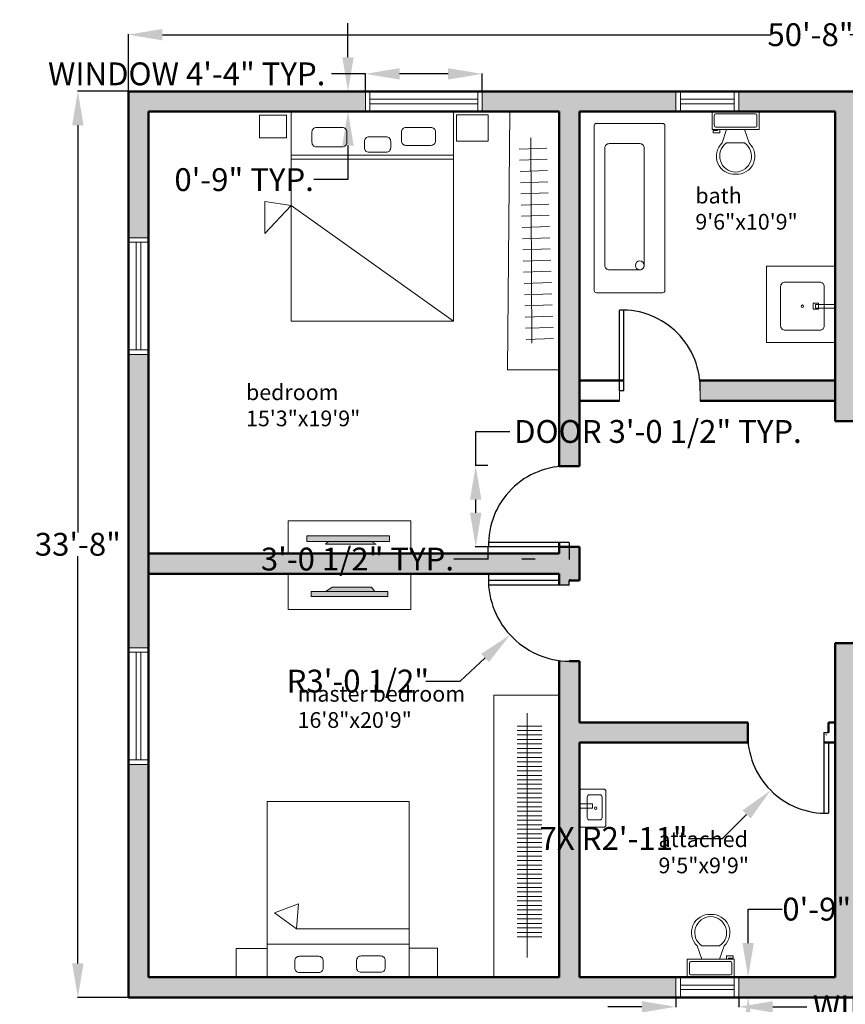
# Model space of a CAD drawing. Units: inches. Extents: x -2 to 7298, y -2 to 4583.
# Tile 4 of 6: x 6016 to 6384, y 4144 to 4583. Entities that reach past the tile are written whole.
import ezdxf

# ---------------------------------------------------------------- set-up
doc = ezdxf.new("R2010")
doc.units = ezdxf.units.IN
doc.header["$MEASUREMENT"] = 0
doc.linetypes.add('ACAD_ISO02W100', pattern=[15, 12, -3])
for name, color, linetype, lineweight in [('A-ANNO-DIMS', 2, 'Continuous', 18), ('A-AREA-IDEN', 7, 'Continuous', 18), ('A-DOOR', 4, 'Continuous', 25), ('A-FLOR-CASE', 30, 'Continuous', 18), ('A-FLOR-FIXT', 9, 'Continuous', 18), ('A-FURN', 8, 'Continuous', 18), ('A-FURN-PATT', 18, 'Continuous', 13), ('A-GLAZ', 4, 'Continuous', 18), ('A-WALL', 7, 'Continuous', 50), ('A-WALL-HIDN', 7, 'ACAD_ISO02W100', 18), ('A-WALL-PATT', 18, 'Continuous', 13)]:
    doc.layers.add(name, color=color, linetype=linetype, lineweight=lineweight)
doc.styles.get("Standard").update_dxf_attribs({"font": 'arial.ttf'})
doc.dimstyles.get("Standard").update_dxf_attribs({"dimtxt": 10.18, "dimasz": 15.18, "dimexe": 0.18, "dimexo": 0.0625, "dimgap": 0.09, "dimtad": 0, "dimtih": 1, "dimtoh": 1, "dimdec": 0, "dimzin": 0, "dimdsep": 46, "dimlunit": 3, "dimtxsty": 'Standard', "dimcen": 0.09, "dimadec": 0, "dimazin": 0, "dimtfac": 1, "dimtdec": 0, "dimtofl": 0, "dimtmove": 0, "dimatfit": 3, "dimfxl": 1, "dimtolj": 1, "dimtzin": 0, "dimarcsym": 0})

# ---------------------------------------------------------------- blocks, each defined once
blk = doc.blocks.new('*U4')
for p, q in [((9.5, -6), (9.5, -2)), ((-10, -8.5), (-8, -8.5)), ((-10, -9.5), (-10, -8.5)), ((-8, -8.5), (-8, -8)), ((-7, -8), (-7, -9.5)), ((-4, -8), (-6, -14)), ((4, -8), (6, -14)), ((-7, -9.5), (-10, -9.5)), ((4, -14), (-4, -14))]:
    blk.add_line(p, q)
blk.add_lwpolyline([(10.5, -8), (10.5, 0), (-10.5, 0), (-10.5, -8)], close=True)
for points in [[(-9.5, -2), (-9.5, -6)], [(8.5, -1), (-8.5, -1)], [(-8.5, -7), (8.5, -7)]]:
    blk.add_lwpolyline(points)
for centre, radius, start, end in [((-8.625, -1.875), 0.8839, 81.8699, 188.1301), ((8.625, -1.875), 0.8839, 351.8699, 98.1301), ((-8.625, -6.125), 0.8839, 171.869898, 278.1301), ((8.625, -6.125), 0.8839, 261.8699, 8.1301), ((-0.4772, -19.9188), 8.0953, 133.01722, 273.38), ((0.0374, -19.8731), 7.127, 124.50543, 269.7), ((-0.0373, -19.8731), 7.127, 270.3, 55.4946), ((0.4773, -19.9188), 8.0953, 266.62, 46.9828)]:
    blk.add_arc(centre, radius, start, end)
blk = doc.blocks.new('*D5')
at = {"layer": 'A-ANNO-DIMS', "color": 0, "lineweight": -2, "transparency": 16777216}
for p, q in [((6064.27, 4551.54), (6064.27, 4576.93)), ((6079.45, 4576.75), (6350.69, 4576.75)), ((6657.09, 4576.75), (6385.84, 4576.75)), ((6672.27, 4551.54), (6672.27, 4576.93))]:
    blk.add_line(p, q, dxfattribs=at)
at = {"layer": 'A-ANNO-DIMS', "color": 0, "transparency": 16777216}
for points in [[(6079.45, 4579.28), (6079.45, 4574.22), (6064.27, 4576.75)], [(6657.09, 4579.28), (6657.09, 4574.22), (6672.27, 4576.75)]]:
    blk.add_solid(points, dxfattribs=at)
at = {"layer": 'Defpoints', "color": 0, "transparency": 16777216}
for p in [(6672.27, 4576.75), (6064.27, 4551.48), (6672.27, 4551.48)]:
    blk.add_point(p, dxfattribs=at)
at = {"layer": 'A-ANNO-DIMS', "color": 0, "transparency": 16777216, "insert": (6368.27, 4576.75), "char_height": 10.18, "attachment_point": 5}
blk.add_mtext('\\A1;50\'-8"', dxfattribs=at)
blk = doc.blocks.new('*D6')
at = {"layer": 'A-ANNO-DIMS', "color": 0, "lineweight": -2, "transparency": 16777216}
for p, q in [((6064.2, 4551.54), (6041.55, 4551.54)), ((6041.73, 4536.36), (6041.73, 4354.8)), ((6041.73, 4162.66), (6041.73, 4344.22)), ((6064.2, 4147.48), (6041.55, 4147.48))]:
    blk.add_line(p, q, dxfattribs=at)
at = {"layer": 'A-ANNO-DIMS', "color": 0, "transparency": 16777216}
for points in [[(6039.2, 4536.36), (6044.26, 4536.36), (6041.73, 4551.54)], [(6039.2, 4162.66), (6044.26, 4162.66), (6041.73, 4147.48)]]:
    blk.add_solid(points, dxfattribs=at)
at = {"layer": 'Defpoints', "color": 0, "transparency": 16777216}
for p in [(6064.27, 4551.54), (6041.73, 4147.48), (6064.27, 4147.48)]:
    blk.add_point(p, dxfattribs=at)
at = {"layer": 'A-ANNO-DIMS', "color": 0, "transparency": 16777216, "insert": (6041.73, 4349.51), "char_height": 10.18, "attachment_point": 5}
blk.add_mtext('\\A1;33\'-8"', dxfattribs=at)
blk = doc.blocks.new('WINDOW-48IN')
for p, q in [((-2, 4.5), (-2, -4.5)), ((0, 4.5), (0, -4.5)), ((48, 4.5), (48, -4.5)), ((50, 4.5), (50, -4.5)), ((0, 1), (48, 1)), ((0, -1), (48, -1))]:
    blk.add_line(p, q)
blk = doc.blocks.new('WINDOW-24IN')
for p, q in [((-26, 4.5), (-26, -4.5)), ((-24, 4.5), (-24, -4.5)), ((0, 4.5), (0, -4.5)), ((2, 4.5), (2, -4.5)), ((-24, 1), (0, 1)), ((-24, -1), (0, -1))]:
    blk.add_line(p, q)
blk = doc.blocks.new('DOOR-SWING-36IN')
for p, q in [((0, 0), (0, 36)), ((2, 0), (2, 36)), ((2, 0), (0, 0))]:
    blk.add_line(p, q)
blk.add_arc((1, 1), 35.01, 358.3634, 91.6366)
blk = doc.blocks.new('*D35')
at = {"layer": 'A-ANNO-DIMS', "color": 0, "lineweight": -2, "transparency": 16777216}
for p, q in [((6169.92, 4559.28), (6154.74, 4559.28)), ((6169.92, 4551.54), (6169.92, 4559.46)), ((6206.74, 4559.28), (6185.1, 4559.28)), ((6221.92, 4551.54), (6221.92, 4559.46))]:
    blk.add_line(p, q, dxfattribs=at)
at = {"layer": 'A-ANNO-DIMS', "color": 0, "transparency": 16777216}
for points in [[(6185.1, 4561.81), (6185.1, 4556.75), (6169.92, 4559.28)], [(6206.74, 4561.81), (6206.74, 4556.75), (6221.92, 4559.28)]]:
    blk.add_solid(points, dxfattribs=at)
at = {"layer": 'Defpoints', "color": 0, "transparency": 16777216}
for p in [(6169.92, 4559.28), (6169.92, 4551.48), (6221.92, 4551.48)]:
    blk.add_point(p, dxfattribs=at)
at = {"layer": 'A-ANNO-DIMS', "color": 0, "transparency": 16777216, "insert": (6090.24, 4559.28), "char_height": 10.18, "attachment_point": 5}
blk.add_mtext('\\A1;WINDOW 4\'-4" TYP.', dxfattribs=at)
blk = doc.blocks.new('*D36')
at = {"layer": 'A-ANNO-DIMS', "color": 0, "lineweight": -2, "transparency": 16777216}
for p, q in [((6162.12, 4566.66), (6162.12, 4581.84)), ((6169.86, 4551.48), (6161.94, 4551.48)), ((6169.86, 4542.48), (6161.94, 4542.48)), ((6162.12, 4527.3), (6162.12, 4512.12)), ((6162.12, 4512.12), (6146.94, 4512.12))]:
    blk.add_line(p, q, dxfattribs=at)
at = {"layer": 'A-ANNO-DIMS', "color": 0, "transparency": 16777216}
for points in [[(6159.59, 4566.66), (6164.65, 4566.66), (6162.12, 4551.48)], [(6159.59, 4527.3), (6164.65, 4527.3), (6162.12, 4542.48)]]:
    blk.add_solid(points, dxfattribs=at)
at = {"layer": 'Defpoints', "color": 0, "transparency": 16777216}
for p in [(6169.92, 4551.48), (6162.12, 4542.48), (6169.92, 4542.48)]:
    blk.add_point(p, dxfattribs=at)
at = {"layer": 'A-ANNO-DIMS', "color": 0, "transparency": 16777216, "insert": (6115.83, 4512.12), "char_height": 10.18, "attachment_point": 5}
blk.add_mtext('\\A1;0\'-9" TYP.', dxfattribs=at)
blk = doc.blocks.new('*D39')
at = {"layer": 'A-ANNO-DIMS', "color": 0, "lineweight": -2, "transparency": 16777216}
for p, q in [((6308.27, 4147.41), (6308.27, 4143.1)), ((6336.27, 4147.41), (6336.27, 4143.1)), ((6293.09, 4143.28), (6277.91, 4143.28)), ((6351.45, 4143.28), (6366.63, 4143.28))]:
    blk.add_line(p, q, dxfattribs=at)
at = {"layer": 'A-ANNO-DIMS', "color": 0, "transparency": 16777216}
for points in [[(6293.09, 4145.81), (6293.09, 4140.75), (6308.27, 4143.28)], [(6351.45, 4145.81), (6351.45, 4140.75), (6336.27, 4143.28)]]:
    blk.add_solid(points, dxfattribs=at)
at = {"layer": 'Defpoints', "color": 0, "transparency": 16777216}
for p in [(6308.27, 4147.48), (6336.27, 4147.48), (6336.27, 4143.28)]:
    blk.add_point(p, dxfattribs=at)
at = {"layer": 'A-ANNO-DIMS', "color": 0, "transparency": 16777216, "insert": (6431.13, 4143.28), "char_height": 10.18, "attachment_point": 5}
blk.add_mtext('\\A1;WINDOW 2\'-4" TYP.', dxfattribs=at)
blk = doc.blocks.new('*D40')
at = {"layer": 'A-ANNO-DIMS', "color": 0, "lineweight": -2, "transparency": 16777216}
for p, q in [((6340.47, 4171.66), (6340.47, 4186.84)), ((6340.47, 4186.84), (6355.65, 4186.84)), ((6336.33, 4156.48), (6340.65, 4156.48)), ((6336.33, 4147.48), (6340.65, 4147.48)), ((6340.47, 4132.3), (6340.47, 4117.12))]:
    blk.add_line(p, q, dxfattribs=at)
at = {"layer": 'A-ANNO-DIMS', "color": 0, "transparency": 16777216}
for points in [[(6337.94, 4171.66), (6343, 4171.66), (6340.47, 4156.48)], [(6337.94, 4132.3), (6343, 4132.3), (6340.47, 4147.48)]]:
    blk.add_solid(points, dxfattribs=at)
at = {"layer": 'Defpoints', "color": 0, "transparency": 16777216}
for p in [(6336.27, 4156.48), (6340.47, 4156.48), (6336.27, 4147.48)]:
    blk.add_point(p, dxfattribs=at)
at = {"layer": 'A-ANNO-DIMS', "color": 0, "transparency": 16777216, "insert": (6386.76, 4186.84), "char_height": 10.18, "attachment_point": 5}
blk.add_mtext('\\A1;0\'-9" TYP.', dxfattribs=at)
blk = doc.blocks.new('*D41')
at = {"layer": 'A-ANNO-DIMS', "color": 0, "lineweight": -2, "transparency": 16777216}
for p, q in [((6219.05, 4384.64), (6219.05, 4399.82)), ((6219.05, 4399.82), (6234.23, 4399.82)), ((6224.43, 4384.64), (6218.87, 4384.64)), ((6219.05, 4363.54), (6219.05, 4369.46)), ((6224.43, 4348.36), (6218.87, 4348.36))]:
    blk.add_line(p, q, dxfattribs=at)
at = {"layer": 'A-ANNO-DIMS', "color": 0, "transparency": 16777216}
for points in [[(6216.52, 4369.46), (6221.58, 4369.46), (6219.05, 4384.64)], [(6216.52, 4363.54), (6221.58, 4363.54), (6219.05, 4348.36)]]:
    blk.add_solid(points, dxfattribs=at)
at = {"layer": 'Defpoints', "color": 0, "transparency": 16777216}
for p in [(6219.05, 4384.64), (6224.49, 4384.64), (6224.49, 4348.36)]:
    blk.add_point(p, dxfattribs=at)
at = {"layer": 'A-ANNO-DIMS', "color": 0, "transparency": 16777216, "insert": (6300.26, 4399.82), "char_height": 10.18, "attachment_point": 5}
blk.add_mtext('\\A1;DOOR 3\'-0 1/2" TYP.', dxfattribs=at)
blk = doc.blocks.new('*D42')
at = {"layer": 'A-ANNO-DIMS', "color": 0, "lineweight": -2, "transparency": 16777216}
for p, q in [((6224.49, 4348.3), (6224.49, 4342.74)), ((6260.77, 4348.3), (6260.77, 4342.74)), ((6224.49, 4342.92), (6209.31, 4342.92)), ((6245.59, 4342.92), (6239.67, 4342.92))]:
    blk.add_line(p, q, dxfattribs=at)
at = {"layer": 'A-ANNO-DIMS', "color": 0, "transparency": 16777216}
for points in [[(6239.67, 4345.45), (6239.67, 4340.39), (6224.49, 4342.92)], [(6245.59, 4345.45), (6245.59, 4340.39), (6260.77, 4342.92)]]:
    blk.add_solid(points, dxfattribs=at)
at = {"layer": 'Defpoints', "color": 0, "transparency": 16777216}
for p in [(6224.49, 4348.36), (6260.77, 4348.36), (6224.49, 4342.92)]:
    blk.add_point(p, dxfattribs=at)
at = {"layer": 'A-ANNO-DIMS', "color": 0, "transparency": 16777216, "insert": (6166.34, 4342.92), "char_height": 10.18, "attachment_point": 5}
blk.add_mtext('\\A1;3\'-0 1/2" TYP.', dxfattribs=at)
blk = doc.blocks.new('*D66')
at = {"layer": 'A-ANNO-DIMS', "color": 0, "lineweight": -2, "transparency": 16777216}
for p, q in [((6030.986562, 4134.626544), (6015.806562, 4134.626544)), ((6046.166562, 4097.966533), (6046.166562, 4134.806544)), ((6112.578072, 4097.966533), (6112.578072, 4134.806544)), ((6127.758072, 4134.626544), (6142.938072, 4134.626544))]:
    blk.add_line(p, q, dxfattribs=at)
at = {"layer": 'A-ANNO-DIMS', "color": 0, "transparency": 16777216}
for points in [[(6030.986562, 4137.156544), (6030.986562, 4132.096544), (6046.166562, 4134.626544)], [(6127.758072, 4137.156544), (6127.758072, 4132.096544), (6112.578072, 4134.626544)]]:
    blk.add_solid(points, dxfattribs=at)
at = {"layer": 'Defpoints', "color": 0, "transparency": 16777216}
for p in [(6112.578072, 4134.626544), (6046.166562, 4097.904033), (6112.578072, 4097.904033)]:
    blk.add_point(p, dxfattribs=at)
at = {"layer": 'A-ANNO-DIMS', "color": 0, "transparency": 16777216, "insert": (6079.372317, 4134.626544), "char_height": 10.18, "attachment_point": 5}
blk.add_mtext('\\A1;5\'-6 1/2"', dxfattribs=at)
blk = doc.blocks.new('*D92')
at = {"layer": 'A-ANNO-DIMS', "color": 0, "lineweight": -2, "transparency": 16777216}
for p, q in [((6261.09, 4333.86), (6261.27, 4333.86)), ((6261.18, 4333.77), (6261.18, 4333.95)), ((6212.05, 4288.51), (6223.21, 4298.81)), ((6196.87, 4288.51), (6212.05, 4288.51))]:
    blk.add_line(p, q, dxfattribs=at)
at = {"layer": 'A-ANNO-DIMS', "color": 0, "transparency": 16777216}
blk.add_solid([(6221.49, 4300.67), (6224.92, 4296.95), (6234.36, 4309.1)], dxfattribs=at)
at = {"layer": 'Defpoints', "color": 0, "transparency": 16777216}
for p in [(6261.18, 4333.86), (6234.36, 4309.1)]:
    blk.add_point(p, dxfattribs=at)
at = {"layer": 'A-ANNO-DIMS', "color": 0, "transparency": 16777216, "insert": (6166.52, 4288.51), "char_height": 10.18, "attachment_point": 5}
blk.add_mtext('\\A1;R3\'-0 1/2"', dxfattribs=at)
blk = doc.blocks.new('*D93')
at = {"layer": 'A-ANNO-DIMS', "color": 0, "lineweight": -2, "transparency": 16777216}
for p, q in [((6375.18, 4264.57), (6375.36, 4264.57)), ((6375.27, 4264.48), (6375.27, 4264.66)), ((6329.04, 4218.34), (6339.77, 4229.08)), ((6313.86, 4218.34), (6329.04, 4218.34))]:
    blk.add_line(p, q, dxfattribs=at)
at = {"layer": 'A-ANNO-DIMS', "color": 0, "transparency": 16777216}
blk.add_solid([(6337.99, 4230.87), (6341.56, 4227.29), (6350.51, 4239.81)], dxfattribs=at)
at = {"layer": 'Defpoints', "color": 0, "transparency": 16777216}
for p in [(6375.27, 4264.57), (6350.51, 4239.81)]:
    blk.add_point(p, dxfattribs=at)
at = {"layer": 'A-ANNO-DIMS', "color": 0, "transparency": 16777216, "insert": (6280.52, 4218.34), "char_height": 10.18, "attachment_point": 5}
blk.add_mtext('\\A1;7X R2\'-11"', dxfattribs=at)

msp = doc.modelspace()

# ---------------------------------------------------------------- hatches: boundary and pattern name
at = {"layer": 'A-FURN-PATT'}
h = msp.add_hatch(color=256, dxfattribs=at)
h.dxf.hatch_style = 1
h.paths.add_polyline_path([(6180.61, 4353.29), (6143.73, 4353.29), (6143.73, 4350.76), (6180.61, 4350.76)])
h.paths.add_polyline_path([(6172.61, 4350.76), (6153.4, 4350.76), (6152.16, 4349.62), (6174.65, 4349.62)])
h = msp.add_hatch(color=256, dxfattribs=at)
h.dxf.hatch_style = 1
h.paths.add_polyline_path([(6179.95, 4328.53), (6145.73, 4328.53), (6145.73, 4326.18), (6179.95, 4326.18)])
h.paths.add_polyline_path([(6172.57, 4330.32), (6155.12, 4330.32), (6152.28, 4328.53), (6174.06, 4328.53)])
at = {"layer": 'A-WALL-PATT'}
h = msp.add_hatch(color=256, dxfattribs=at)
h.dxf.hatch_style = 1
h.paths.add_polyline_path([(6073.27, 4434.19), (6064.27, 4434.19), (6064.27, 4303.39), (6073.27, 4303.39), (6073.27, 4305.48)])
h.paths.add_polyline_path([(6265.27, 4348.36), (6256.27, 4348.36), (6256.27, 4345.36), (6073.27, 4345.36), (6073.27, 4336.36), (6256.27, 4336.36), (6256.27, 4331.36), (6260.77, 4331.36), (6260.77, 4333.36), (6265.27, 4333.36)])
h.paths.add_polyline_path([(6073.27, 4251.39), (6064.27, 4251.39), (6064.27, 4147.48), (6308.27, 4147.48), (6308.27, 4156.48), (6265.27, 4156.48), (6265.27, 4256.48), (6265.27, 4261.07), (6340.27, 4261.07), (6340.27, 4263.57, -0.014283), (6340.27, 4265.57), (6340.27, 4270.07), (6265.27, 4270.07), (6265.27, 4297.36), (6261.6, 4297.36, -0.036646), (6256.27, 4297.69), (6256.27, 4156.48), (6073.27, 4156.48)])
h.paths.add_polyline_path([(6422.77, 4156.48), (6388.27, 4156.48), (6388.27, 4305.48), (6379.27, 4305.48), (6379.27, 4270.07), (6379.27, 4261.07), (6379.27, 4156.48), (6336.27, 4156.48), (6336.27, 4147.48), (6422.77, 4147.48)])
h.paths.add_polyline_path([(6552.77, 4156.48), (6518.27, 4156.48), (6518.27, 4261.05), (6509.27, 4261.05), (6509.27, 4156.48), (6474.77, 4156.48), (6474.77, 4147.48), (6552.77, 4147.48)])
h.paths.add_polyline_path([(6672.27, 4252.66), (6663.27, 4252.66), (6663.27, 4156.48), (6628.77, 4156.48), (6628.77, 4147.48), (6672.27, 4147.48)])
h.paths.add_polyline_path([(6672.27, 4385.98), (6663.27, 4385.98), (6663.27, 4305.48), (6561.68, 4305.48, -0.01877), (6561.79, 4302.48), (6561.79, 4296.48), (6663.27, 4296.48), (6663.27, 4287.22), (6672.27, 4287.22)])
h.paths.add_polyline_path([(6518.27, 4542.48), (6663.27, 4542.48), (6663.27, 4461.98), (6672.27, 4461.98), (6672.27, 4551.48), (6336.27, 4551.48), (6336.27, 4542.48), (6379.27, 4542.48), (6379.27, 4404.48), (6388.27, 4404.48), (6388.27, 4506.48), (6388.27, 4542.48), (6509.27, 4542.48), (6509.27, 4413.48), (6509.27, 4404.48), (6509.27, 4305.48), (6518.27, 4305.48)])
h.paths.add_polyline_path([(6379.27, 4422.48), (6319.12, 4422.48), (6319.12, 4419.98, -0.014283), (6319.12, 4417.98), (6319.12, 4413.48), (6379.27, 4413.48)])
h.paths.add_polyline_path([(6265.27, 4542.48), (6308.27, 4542.48), (6308.27, 4551.48), (6221.92, 4551.48), (6221.92, 4542.48), (6256.27, 4542.48), (6256.27, 4384.36), (6258.77, 4384.36, -0.014283), (6260.77, 4384.36), (6265.27, 4384.36)])
h.paths.add_polyline_path([(6169.92, 4551.48), (6064.27, 4551.48), (6064.27, 4486.19), (6073.27, 4486.19), (6073.27, 4542.48), (6169.92, 4542.48)])

# ---------------------------------------------------------------- linework, layer by layer
at = {"layer": 'A-DOOR'}
for p, q in [((6256.27, 4333.36), (6224.77, 4333.36)), ((6260.77, 4331.36), (6260.77, 4333.36)), ((6260.77, 4331.36), (6224.77, 4331.36)), ((6374.27, 4265.57), (6374.27, 4229.57)), ((6374.27, 4265.57), (6376.27, 4265.57)), ((6376.27, 4261.07), (6376.27, 4229.57))]:
    msp.add_line(p, q, dxfattribs=at)
for centre, radius, start, end in [((6261.18, 4333.86), 36.5, 176.0728, 269.346), ((6375.27, 4264.57), 35.01, 178.3634, 271.6366)]:
    msp.add_arc(centre, radius, start, end, dxfattribs=at)
at = {"layer": 'A-FLOR-CASE'}
for p, q in [((6234.29, 4542.48), (6233.25, 4427.35)), ((6243.67, 4530.72), (6244.02, 4439.15)), ((6238.44, 4525.75), (6250.68, 4526.19)), ((6238.62, 4520.76), (6250.85, 4521.19)), ((6238.8, 4515.76), (6251.03, 4516.2)), ((6238.98, 4510.76), (6251.21, 4511.2)), ((6239.16, 4505.77), (6251.39, 4506.2)), ((6239.34, 4500.77), (6251.57, 4501.21)), ((6239.51, 4495.77), (6251.75, 4496.21)), ((6239.69, 4490.78), (6251.92, 4491.21)), ((6239.87, 4485.78), (6252.1, 4486.22)), ((6240.05, 4480.78), (6252.28, 4481.22)), ((6240.23, 4475.79), (6252.46, 4476.22)), ((6240.41, 4470.79), (6252.64, 4471.23)), ((6240.58, 4465.79), (6252.81, 4466.23)), ((6240.76, 4460.8), (6252.99, 4461.23)), ((6240.94, 4455.8), (6253.17, 4456.24)), ((6241.12, 4450.8), (6253.35, 4451.24)), ((6241.3, 4445.81), (6253.53, 4446.24)), ((6241.47, 4440.81), (6253.71, 4441.25)), ((6233.25, 4427.35), (6256.27, 4427.35)), ((6256.27, 4282.25), (6227.05, 4282.25)), ((6227.05, 4282.25), (6227.05, 4156.48)), ((6241.97, 4274.22), (6241.97, 4165.31)), ((6237.54, 4268.48), (6248.51, 4268.48)), ((6237.54, 4266.48), (6248.51, 4266.48)), ((6237.54, 4264.48), (6248.51, 4264.48)), ((6237.54, 4262.48), (6248.51, 4262.48)), ((6237.54, 4260.48), (6248.51, 4260.48)), ((6237.54, 4258.48), (6248.51, 4258.48)), ((6237.54, 4256.48), (6248.51, 4256.48)), ((6237.54, 4254.48), (6248.51, 4254.48)), ((6237.54, 4252.48), (6248.51, 4252.48)), ((6237.54, 4250.48), (6248.51, 4250.48)), ((6237.54, 4248.48), (6248.51, 4248.48)), ((6237.54, 4246.48), (6248.51, 4246.48)), ((6237.54, 4244.48), (6248.51, 4244.48)), ((6237.54, 4242.48), (6248.51, 4242.48)), ((6237.54, 4240.48), (6248.51, 4240.48)), ((6237.54, 4238.48), (6248.51, 4238.48)), ((6237.54, 4236.48), (6248.51, 4236.48)), ((6237.54, 4234.48), (6248.51, 4234.48)), ((6237.54, 4232.48), (6248.51, 4232.48)), ((6237.54, 4230.48), (6248.51, 4230.48)), ((6237.54, 4228.48), (6248.51, 4228.48)), ((6237.54, 4226.48), (6248.51, 4226.48)), ((6237.54, 4224.48), (6248.51, 4224.48)), ((6237.54, 4222.48), (6248.51, 4222.48)), ((6237.54, 4220.48), (6248.51, 4220.48)), ((6237.54, 4218.48), (6248.51, 4218.48)), ((6237.54, 4216.48), (6248.51, 4216.48)), ((6237.54, 4214.48), (6248.51, 4214.48)), ((6237.54, 4212.48), (6248.51, 4212.48)), ((6237.54, 4210.48), (6248.51, 4210.48)), ((6237.54, 4208.48), (6248.51, 4208.48)), ((6237.54, 4206.48), (6248.51, 4206.48)), ((6237.54, 4204.48), (6248.51, 4204.48)), ((6237.54, 4202.48), (6248.51, 4202.48)), ((6237.54, 4200.48), (6248.51, 4200.48)), ((6237.54, 4198.48), (6248.51, 4198.48)), ((6237.54, 4196.48), (6248.51, 4196.48)), ((6237.54, 4194.48), (6248.51, 4194.48)), ((6237.54, 4192.48), (6248.51, 4192.48)), ((6237.54, 4190.48), (6248.51, 4190.48)), ((6237.54, 4188.48), (6248.51, 4188.48)), ((6237.54, 4186.48), (6248.51, 4186.48)), ((6237.54, 4184.48), (6248.51, 4184.48)), ((6237.54, 4182.48), (6248.51, 4182.48)), ((6237.54, 4180.48), (6248.51, 4180.48)), ((6237.54, 4178.48), (6248.51, 4178.48)), ((6237.54, 4176.48), (6248.51, 4176.48)), ((6237.54, 4174.48), (6248.51, 4174.48))]:
    msp.add_line(p, q, dxfattribs=at)
at = {"layer": 'A-FLOR-FIXT'}
for p, q in [((6379.27, 4456.45), (6370.45, 4456.45)), ((6370.45, 4456.45), (6370.45, 4454.87)), ((6370.45, 4454.87), (6379.27, 4454.87)), ((6265.27, 4233.71), (6265.27, 4233.71))]:
    msp.add_line(p, q, dxfattribs=at)
for points in [[(6271.87, 4536.16, -0.414214), (6272.87, 4537.16), (6302.4, 4537.16, -0.414214), (6303.4, 4536.16), (6303.4, 4462.68, -0.414214), (6302.4, 4461.68), (6272.87, 4461.68, -0.414214), (6271.87, 4462.68)], [(6276.57, 4526.16, -0.414214), (6278.57, 4528.16), (6292.19, 4528.16, -0.414214), (6294.19, 4526.16), (6294.19, 4473.84, -0.414214), (6292.19, 4471.84), (6278.57, 4471.84, -0.414214), (6276.57, 4473.84)], [(6354.95, 4464.41, -0.414214), (6356.95, 4466.41), (6372.42, 4466.41, -0.414214), (6374.42, 4464.41), (6374.42, 4446.98, -0.414214), (6372.42, 4444.98), (6356.95, 4444.98, -0.414214), (6354.95, 4446.98)], [(6265.27, 4239.35, -0.414214), (6266.27, 4240.35), (6276.07, 4240.35, -0.414214), (6277.07, 4239.35), (6277.07, 4224.37, -0.414214), (6276.07, 4223.37), (6266.27, 4223.37, -0.414214), (6265.27, 4224.37)], [(6268.72, 4236.81, -0.414214), (6269.72, 4237.81), (6274.37, 4237.81, -0.414214), (6275.37, 4236.81), (6275.37, 4227.61, -0.414214), (6274.37, 4226.61), (6269.72, 4226.61, -0.414214), (6268.72, 4227.61)]]:
    msp.add_lwpolyline(points, format="xyb", close=True, dxfattribs=at)
for points in [[(6379.27, 4473.48), (6379.27, 4473.48), (6348.59, 4473.48), (6348.59, 4473.48), (6348.59, 4439.42), (6348.59, 4439.42), (6379.27, 4439.42), (6379.27, 4439.42)], [(6369.44, 4456.99), (6369.44, 4456.99), (6371.82, 4456.99), (6371.82, 4456.99), (6371.82, 4454.31), (6371.82, 4454.31), (6369.44, 4454.31), (6369.44, 4454.31)], [(6265.27, 4233.71), (6265.27, 4233.71), (6271.17, 4233.71), (6271.17, 4233.71), (6271.17, 4231.86), (6271.17, 4231.86), (6265.27, 4231.86), (6265.27, 4231.86)]]:
    msp.add_lwpolyline(points, close=True, dxfattribs=at)
for centre, radius in [((6292.19, 4473.84), 2), ((6364.68, 4455.69), 0.525), ((6272.48, 4231.86), 0.544)]:
    msp.add_circle(centre, radius, dxfattribs=at)
at = {"layer": 'A-FURN'}
for p, q in [((6136.73, 4522.96), (6209.1, 4522.96)), ((6136.73, 4521.27), (6209.1, 4521.27)), ((6136.73, 4500.65), (6125.01, 4502.35)), ((6125.01, 4502.35), (6125.01, 4488.07)), ((6125.01, 4488.07), (6136.73, 4500.65)), ((6209.1, 4449), (6136.73, 4500.65)), ((6153.4, 4350.76), (6152.16, 4349.62)), ((6152.16, 4349.62), (6174.65, 4349.62)), ((6174.65, 4349.62), (6172.61, 4350.76)), ((6152.28, 4328.53), (6155.12, 4330.32)), ((6155.12, 4330.32), (6172.57, 4330.32)), ((6172.57, 4330.32), (6174.06, 4328.53)), ((6129.4, 4185.18), (6140.08, 4189.15)), ((6140.08, 4189.15), (6139.19, 4177.99)), ((6139.19, 4177.99), (6129.4, 4185.18)), ((6189.34, 4177.99), (6139.19, 4177.99)), ((6189.34, 4171.17), (6126.16, 4171.17))]:
    msp.add_line(p, q, dxfattribs=at)
for points in [[(6134.69, 4540.91), (6134.69, 4540.91), (6122.69, 4540.91), (6122.69, 4540.91), (6122.69, 4530.72), (6122.69, 4530.72), (6134.69, 4530.72), (6134.69, 4530.72)], [(6136.73, 4542.48), (6136.73, 4542.48), (6209.1, 4542.48), (6209.1, 4542.48), (6209.1, 4449), (6209.1, 4449), (6136.73, 4449), (6136.73, 4449)], [(6210.54, 4541.05), (6210.54, 4541.05), (6224.56, 4541.05), (6224.56, 4541.05), (6224.56, 4529.31), (6224.56, 4529.31), (6210.54, 4529.31), (6210.54, 4529.31)], [(6135.43, 4345.36), (6135.43, 4345.36), (6190.17, 4345.36), (6190.17, 4345.36), (6190.17, 4359.97), (6190.17, 4359.97), (6135.43, 4359.97), (6135.43, 4359.97)], [(6143.73, 4350.76), (6143.73, 4350.76), (6180.61, 4350.76), (6180.61, 4350.76), (6180.61, 4353.29), (6180.61, 4353.29), (6143.73, 4353.29), (6143.73, 4353.29)], [(6135.42, 4336.36), (6135.42, 4336.36), (6190.17, 4336.36), (6190.17, 4336.36), (6190.17, 4320.4), (6190.17, 4320.4), (6135.42, 4320.4), (6135.42, 4320.4)], [(6145.73, 4328.53), (6145.73, 4328.53), (6179.95, 4328.53), (6179.95, 4328.53), (6179.95, 4326.18), (6179.95, 4326.18), (6145.73, 4326.18), (6145.73, 4326.18)], [(6126.16, 4234.84), (6126.16, 4234.84), (6189.34, 4234.84), (6189.34, 4234.84), (6189.34, 4156.48), (6189.34, 4156.48), (6126.16, 4156.48), (6126.16, 4156.48)], [(6126.16, 4169.34), (6126.16, 4169.34), (6112.21, 4169.34), (6112.21, 4169.34), (6112.21, 4156.48), (6112.21, 4156.48), (6126.16, 4156.48), (6126.16, 4156.48)], [(6189.34, 4169.44), (6189.34, 4169.44), (6202.03, 4169.44), (6202.03, 4169.44), (6202.03, 4156.48), (6202.03, 4156.48), (6189.34, 4156.48), (6189.34, 4156.48)]]:
    msp.add_lwpolyline(points, close=True, dxfattribs=at)
for points in [[(6161.58, 4533.36, 0.414214), (6159.58, 4535.36), (6148.07, 4535.36, 0.414214), (6146.07, 4533.36), (6146.07, 4528.75, 0.414214), (6148.07, 4526.75), (6159.58, 4526.75, 0.414214), (6161.58, 4528.75)], [(6185.95, 4533.36, -0.414214), (6187.95, 4535.36), (6199.09, 4535.36, -0.414214), (6201.09, 4533.36), (6201.09, 4529.37, -0.414214), (6199.09, 4527.37), (6187.95, 4527.37, -0.414214), (6185.95, 4529.37)], [(6169.46, 4529.18, -0.414214), (6171.46, 4531.18), (6179.15, 4531.18, -0.414214), (6181.15, 4529.18), (6181.15, 4526.29, -0.414214), (6179.15, 4524.29), (6171.46, 4524.29, -0.414214), (6169.46, 4526.29)], [(6138.41, 4163.82, -0.414214), (6140.41, 4165.82), (6149.12, 4165.82, -0.414214), (6151.12, 4163.82), (6151.12, 4160.52, -0.414214), (6149.12, 4158.52), (6140.41, 4158.52, -0.414214), (6138.41, 4160.52)], [(6165.96, 4163.96, -0.414214), (6167.96, 4165.96), (6176.67, 4165.96, -0.414214), (6178.67, 4163.96), (6178.67, 4160.65, -0.414214), (6176.67, 4158.65), (6167.96, 4158.65, -0.414214), (6165.96, 4160.65)]]:
    msp.add_lwpolyline(points, format="xyb", close=True, dxfattribs=at)
at = {"layer": 'A-WALL'}
for p, q in [((6672.27, 4551.48), (6064.27, 4551.48)), ((6064.27, 4147.48), (6064.27, 4551.48)), ((6256.27, 4542.48), (6073.27, 4542.48)), ((6073.27, 4305.48), (6073.27, 4542.48)), ((6256.27, 4384.2), (6256.27, 4542.48)), ((6379.27, 4542.48), (6265.27, 4542.48)), ((6265.27, 4384.36), (6265.27, 4542.48)), ((6379.27, 4404.48), (6379.27, 4542.48)), ((6285.12, 4422.48), (6265.27, 4422.48)), ((6379.27, 4422.48), (6318.95, 4422.48)), ((6283.12, 4413.48), (6265.27, 4413.48)), ((6379.27, 4413.48), (6319.12, 4413.48)), ((6379.27, 4404.48), (6388.27, 4404.48)), ((6256.27, 4384.36), (6265.27, 4384.36)), ((6256.27, 4345.36), (6256.27, 4350.36)), ((6256.27, 4348.36), (6265.27, 4348.36)), ((6265.27, 4333.36), (6265.27, 4348.36)), ((6256.27, 4345.36), (6073.27, 4345.36)), ((6256.27, 4336.36), (6073.27, 4336.36)), ((6256.27, 4331.36), (6256.27, 4336.36)), ((6260.77, 4333.36), (6265.27, 4333.36)), ((6073.27, 4305.48), (6073.27, 4296.48)), ((6388.27, 4305.48), (6379.27, 4305.48)), ((6379.27, 4270.07), (6379.27, 4305.48)), ((6073.27, 4156.48), (6073.27, 4296.48)), ((6256.27, 4156.48), (6256.27, 4297.69)), ((6260.77, 4297.36), (6265.27, 4297.36)), ((6265.27, 4270.07), (6265.27, 4297.36)), ((6340.27, 4270.07), (6265.27, 4270.07)), ((6340.27, 4270.07), (6340.27, 4261.07)), ((6379.27, 4270.07), (6376.27, 4270.07)), ((6376.27, 4270.07), (6376.27, 4265.57)), ((6379.27, 4270.07), (6379.27, 4261.07)), ((6265.27, 4256.43), (6265.27, 4261.07)), ((6340.43, 4261.07), (6265.27, 4261.07)), ((6379.27, 4261.07), (6374.27, 4261.07)), ((6379.27, 4156.48), (6379.27, 4261.07)), ((6265.27, 4156.48), (6265.27, 4256.48)), ((6073.27, 4156.48), (6256.27, 4156.48)), ((6265.27, 4156.48), (6379.27, 4156.48)), ((6064.27, 4147.48), (6672.27, 4147.48))]:
    msp.add_line(p, q, dxfattribs=at)
at = {"layer": 'A-WALL-HIDN'}
for p, q in [((6283.12, 4422.48), (6283.12, 4413.48)), ((6319.12, 4422.48), (6319.12, 4413.48))]:
    msp.add_line(p, q, dxfattribs=at)

# ---------------------------------------------------------------- block references
at = {"layer": 'A-DOOR'}
msp.add_blockref('DOOR-SWING-36IN', (6283.12, 4417.98), dxfattribs=at)
at = {"layer": 'A-DOOR', "rotation": 90.00000000000146}
msp.add_blockref('DOOR-SWING-36IN', (6260.77, 4348.36), dxfattribs=at)
at = {"layer": 'A-FLOR-FIXT'}
msp.add_blockref('*U4', (6334.87, 4542.48), dxfattribs=at)
at = {"layer": 'A-FLOR-FIXT', "rotation": 180}
msp.add_blockref('*U4', (6323.77, 4156.48), dxfattribs=at)
at = {"layer": 'A-GLAZ'}
for p, rotation in [((6219.92, 4546.98), 180), ((6068.77, 4436.19), 90.0000000000016), ((6068.77, 4301.39), 270.0000000000055)]:
    msp.add_blockref('WINDOW-48IN', p, dxfattribs=dict(at, rotation=rotation))
for p in [(6334.27, 4546.98), (6334.27, 4151.98)]:
    msp.add_blockref('WINDOW-24IN', p, dxfattribs=at)

# ---------------------------------------------------------------- texts
at = {"layer": 'A-AREA-IDEN', "char_height": 7, "attachment_point": 1}
for s, insert in [('bath\\P9\'6"x10\'9"', (6316.93, 4508.49)), ('bedroom\\P15\'3"x19\'9"', (6116.68, 4420.81)), ('master bedroom\\P16\'8"x20\'9"', (6139.65, 4286.34)), ('attached\\P9\'5"x9\'9"', (6300.51, 4221.49))]:
    msp.add_mtext_dynamic_manual_height_columns(s, width=119.0967, gutter_width=1, heights=[0], dxfattribs=dict(at, insert=insert))

# ---------------------------------------------------------------- dimensions: what is measured, and where the dimension line sits
at = {"layer": 'A-ANNO-DIMS'}
for base, p1, p2, angle, text, picture, middle in [((6169.92, 4559.28), (6221.92, 4551.48), (6169.92, 4551.48), 180, 'WINDOW <> TYP.', '*D35', (6090.24, 4559.28)), ((6162.12, 4542.48), (6169.92, 4551.48), (6169.92, 4542.48), 270, '<> TYP.', '*D36', (6115.83, 4512.12)), ((6219.05, 4384.64), (6224.49, 4348.36), (6224.49, 4384.64), 90, 'DOOR <> TYP.', '*D41', (6300.26, 4399.82)), ((6224.49, 4342.92), (6260.77, 4348.36), (6224.49, 4348.36), 180, '<> TYP.', '*D42', (6166.34, 4342.92)), ((6340.47, 4156.48), (6336.27, 4147.48), (6336.27, 4156.48), 90, '<> TYP.', '*D40', (6386.76, 4186.84))]:
    dim = msp.add_linear_dim(base=base, p1=p1, p2=p2, angle=angle, text=text, dimstyle='Standard', override={"dimdec": 1, "dimlfac": 1, "dimrnd": 0, "dimzin": 1, "dimdsep": 46, "dimlunit": 4, "dimfrac": 2}, dxfattribs=at)
    dim.commit()
    dim.dimension.update_dxf_attribs({"geometry": picture, "text_midpoint": middle})
for base, p1, p2, override, picture, middle in [((6672.27, 4576.75), (6064.27, 4551.48), (6672.27, 4551.48), {"dimclrd": 0, "dimclre": 0, "dimclrt": 0}, '*D5', (6368.27, 4576.75)), ((6112.58, 4134.63), (6046.17, 4097.9), (6112.58, 4097.9), {"dimdec": 1, "dimlfac": 1, "dimrnd": 0, "dimzin": 1, "dimdsep": 46, "dimlunit": 4, "dimfrac": 2}, '*D66', (6079.37, 4134.63))]:
    dim = msp.add_linear_dim(base=base, p1=p1, p2=p2, dimstyle='Standard', override=override, dxfattribs=at)
    dim.commit()
    dim.dimension.update_dxf_attribs({"geometry": picture, "text_midpoint": middle})
dim = msp.add_linear_dim(base=(6041.73, 4147.48), p1=(6064.27, 4551.54), p2=(6064.27, 4147.48), angle=90, dimstyle='Standard', override={"dimclrd": 0, "dimclre": 0, "dimclrt": 0}, dxfattribs=at)
dim.commit()
dim.dimension.update_dxf_attribs({"geometry": '*D6', "text_midpoint": (6041.73, 4349.51)})
dim = msp.add_radius_dim(center=(6261.18, 4333.86), mpoint=(6234.36, 4309.1), dimstyle='Standard', override={"dimdec": 1, "dimlfac": 1, "dimrnd": 0, "dimzin": 1, "dimdsep": 46, "dimlunit": 4, "dimfrac": 2}, dxfattribs=at)
dim.commit()
dim.dimension.update_dxf_attribs({"geometry": '*D92', "text_midpoint": (6166.52, 4288.51)})
dim = msp.add_radius_dim(center=(6375.27, 4264.57), mpoint=(6350.51, 4239.81), text='7X <>', dimstyle='Standard', override={"dimdec": 1, "dimlfac": 1, "dimrnd": 0, "dimzin": 1, "dimdsep": 46, "dimlunit": 4, "dimfrac": 2}, dxfattribs=at)
dim.commit()
dim.dimension.update_dxf_attribs({"geometry": '*D93', "text_midpoint": (6280.52, 4218.34)})
dim = msp.add_linear_dim(base=(6336.27, 4143.28), p1=(6308.27, 4147.48), p2=(6336.27, 4147.48), text='WINDOW <> TYP.', dimstyle='Standard', override={"dimdec": 1, "dimlfac": 1, "dimrnd": 0, "dimzin": 1, "dimdsep": 46, "dimlunit": 4, "dimfrac": 2}, dxfattribs=at)
dim.commit()
dim.dimension.update_dxf_attribs({"geometry": '*D39', "text_midpoint": (6431.13, 4143.28)})

doc.saveas('drawing.dxf')
